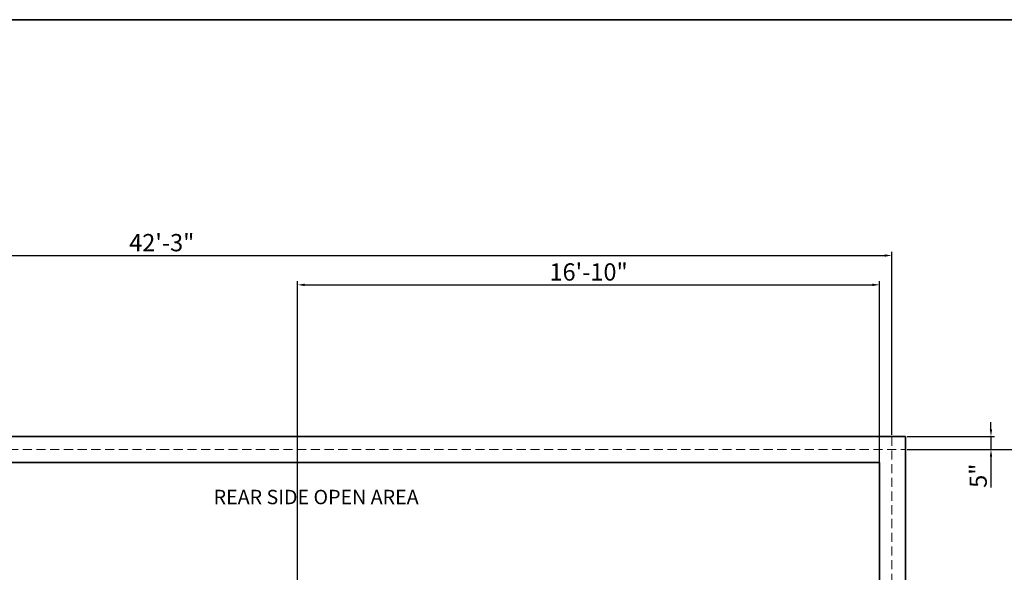
# Model space of a CAD drawing. Units: inches. Extents: x 2123 to 2977, y 1464 to 2698.
# Tile 9 of 10: x 2459 to 2801, y 2506 to 2698. Entities that reach past the tile are written whole.
import ezdxf

# ---------------------------------------------------------------- set-up
doc = ezdxf.new("R2010")
doc.units = ezdxf.units.IN
doc.linetypes.add('HIDDEN2', pattern=[4.7625, 3.175, -1.5875])
for name, color, linetype, lineweight in [('A-ANNO-DIMS', 2, 'Continuous', 18), ('A-ANNO-TTLB', 7, 'Continuous', 35), ('A-AREA-IDEN', 7, 'Continuous', 25), ('C-PROP', 21, 'HIDDEN2', 18), ('L-SITE-WALL', 7, 'Continuous', 35)]:
    doc.layers.add(name, color=color, linetype=linetype, lineweight=lineweight)
doc.styles.get("Standard").update_dxf_attribs({"font": 'arial.ttf'})
doc.dimstyles.new('ISO-25', dxfattribs={"dimtxt": 6, "dimasz": 2.5, "dimexe": 1.25, "dimexo": 0.625, "dimtad": 1, "dimdec": 0, "dimlunit": 3, "dimtxsty": 'Standard', "dimcen": 2.5, "dimadec": 0, "dimazin": 0, "dimtfac": 1, "dimtdec": 0, "dimtmove": 0, "dimatfit": 3, "dimfxl": 1, "dimarcsym": 0})

# ---------------------------------------------------------------- blocks, each defined once
blk = doc.blocks.new('*D9')
at = {"layer": 'A-ANNO-DIMS', "color": 0, "lineweight": -2, "transparency": 16777216}
for p, q in [((2767.56, 2548.37), (2808.58, 2548.37)), ((2807.33, 2545.87), (2807.33, 1686.46)), ((2767.56, 1683.96), (2808.58, 1683.96))]:
    blk.add_line(p, q, dxfattribs=at)
at = {"layer": 'A-ANNO-DIMS', "color": 0, "transparency": 16777216}
for points in [[(2806.91, 2545.87), (2807.74, 2545.87), (2807.33, 2548.37)], [(2806.91, 1686.46), (2807.74, 1686.46), (2807.33, 1683.96)]]:
    blk.add_solid(points, dxfattribs=at)
at = {"layer": 'Defpoints', "color": 0, "transparency": 16777216}
for p in [(2766.94, 2548.37), (2766.94, 1683.96), (2807.33, 1683.96)]:
    blk.add_point(p, dxfattribs=at)
at = {"layer": 'A-ANNO-DIMS', "color": 0, "transparency": 16777216, "insert": (2803.69, 2116.16), "char_height": 6, "attachment_point": 5, "rotation": 90}
blk.add_mtext("72'", dxfattribs=at)
blk = doc.blocks.new('*D10')
at = {"layer": 'A-ANNO-DIMS', "color": 0, "lineweight": -2, "transparency": 16777216}
for p, q in [((2796.59, 2555.37), (2796.59, 2557.87)), ((2767.56, 2552.87), (2797.84, 2552.87)), ((2796.59, 2552.87), (2796.59, 2548.37)), ((2767.56, 2548.37), (2797.84, 2548.37)), ((2796.59, 2545.87), (2796.59, 2535.22))]:
    blk.add_line(p, q, dxfattribs=at)
at = {"layer": 'A-ANNO-DIMS', "color": 0, "transparency": 16777216}
for points in [[(2796.18, 2555.37), (2797.01, 2555.37), (2796.59, 2552.87)], [(2796.18, 2545.87), (2797.01, 2545.87), (2796.59, 2548.37)]]:
    blk.add_solid(points, dxfattribs=at)
at = {"layer": 'Defpoints', "color": 0, "transparency": 16777216}
for p in [(2766.94, 2552.87), (2766.94, 2548.37), (2796.59, 2548.37)]:
    blk.add_point(p, dxfattribs=at)
at = {"layer": 'A-ANNO-DIMS', "color": 0, "transparency": 16777216, "insert": (2792.92, 2539.3), "char_height": 6, "attachment_point": 5, "rotation": 90}
blk.add_mtext('5"', dxfattribs=at)
blk = doc.blocks.new('*D11')
at = {"layer": 'A-ANNO-DIMS', "color": 0, "lineweight": -2, "transparency": 16777216}
for p, q in [((2255.34, 2553.5), (2255.34, 2617)), ((2257.84, 2615.75), (2759.66, 2615.75)), ((2762.16, 2553.5), (2762.16, 2617))]:
    blk.add_line(p, q, dxfattribs=at)
at = {"layer": 'A-ANNO-DIMS', "color": 0, "transparency": 16777216}
for points in [[(2257.84, 2616.16), (2257.84, 2615.33), (2255.34, 2615.75)], [(2759.66, 2616.16), (2759.66, 2615.33), (2762.16, 2615.75)]]:
    blk.add_solid(points, dxfattribs=at)
at = {"layer": 'Defpoints', "color": 0, "transparency": 16777216}
for p in [(2762.16, 2615.75), (2255.34, 2552.87), (2762.16, 2552.87)]:
    blk.add_point(p, dxfattribs=at)
at = {"layer": 'A-ANNO-DIMS', "color": 0, "transparency": 16777216, "insert": (2508.75, 2619.44), "char_height": 6, "attachment_point": 5}
blk.add_mtext('42\'-3"', dxfattribs=at)
blk = doc.blocks.new('*D57')
at = {"layer": 'A-ANNO-DIMS', "color": 0, "lineweight": -2, "transparency": 16777216}
for p, q in [((2555.89, 1805.13), (2555.89, 2606.82)), ((2558.39, 2605.57), (2755.44, 2605.57)), ((2757.94, 1805.13), (2757.94, 2606.82))]:
    blk.add_line(p, q, dxfattribs=at)
at = {"layer": 'A-ANNO-DIMS', "color": 0, "transparency": 16777216}
for points in [[(2558.39, 2605.99), (2558.39, 2605.15), (2555.89, 2605.57)], [(2755.44, 2605.99), (2755.44, 2605.15), (2757.94, 2605.57)]]:
    blk.add_solid(points, dxfattribs=at)
at = {"layer": 'Defpoints', "color": 0, "transparency": 16777216}
for p in [(2757.94, 2605.57), (2555.89, 1804.5), (2757.94, 1804.5)]:
    blk.add_point(p, dxfattribs=at)
at = {"layer": 'A-ANNO-DIMS', "color": 0, "transparency": 16777216, "insert": (2656.91, 2609.26), "char_height": 6, "attachment_point": 5}
blk.add_mtext('16\'-10"', dxfattribs=at)

msp = doc.modelspace()

# ---------------------------------------------------------------- linework, layer by layer
at = {"layer": 'A-ANNO-TTLB'}
msp.add_lwpolyline([(2123.3, 2697.62), (2977.18, 2697.62), (2977.18, 1463.53), (2123.3, 1463.53)], close=True, dxfattribs=at)
at = {"layer": 'C-PROP'}
for p, q in [((2762.16, 2552.87), (2762.16, 1683.96)), ((2250.94, 2548.37), (2766.94, 2548.37))]:
    msp.add_line(p, q, dxfattribs=at)
at = {"layer": 'L-SITE-WALL'}
for p, q in [((2766.94, 2552.87), (2250.94, 2552.87)), ((2766.94, 2425.87), (2766.94, 2552.87)), ((2757.94, 2543.87), (2259.94, 2543.87)), ((2757.94, 2425.87), (2757.94, 2543.87))]:
    msp.add_line(p, q, dxfattribs=at)

# ---------------------------------------------------------------- texts
at = {"layer": 'A-AREA-IDEN', "insert": (2526.77, 2534.41), "char_height": 5, "attachment_point": 1}
msp.add_mtext_dynamic_manual_height_columns('REAR SIDE OPEN AREA', width=209.6107, gutter_width=12.5, heights=[0], dxfattribs=at)

# ---------------------------------------------------------------- dimensions: what is measured, and where the dimension line sits
at = {"layer": 'A-ANNO-DIMS'}
for base, p1, p2, override, picture, middle in [((2762.16, 2615.75), (2255.34, 2552.87), (2762.16, 2552.87), {"dimclrd": 0, "dimclre": 0, "dimclrt": 0}, '*D11', (2508.75, 2619.44)), ((2757.9353, 2605.5708), (2555.8869, 1804.5032), (2757.9353, 1804.5032), {"dimdec": 1, "dimlfac": 1, "dimrnd": 0, "dimzin": 1, "dimdsep": 46, "dimlunit": 4, "dimfrac": 2}, '*D57', (2656.9111, 2609.2592))]:
    dim = msp.add_linear_dim(base=base, p1=p1, p2=p2, dimstyle='ISO-25', override=override, dxfattribs=at)
    dim.commit()
    dim.dimension.update_dxf_attribs({"geometry": picture, "text_midpoint": middle})
for base, p1, p2, picture, middle in [((2796.59419876, 2548.37076072), (2766.93529578, 2552.87076072), (2766.93529578, 2548.37076072), '*D10', (2792.91803914, 2539.29760247)), ((2807.33, 1683.96), (2766.94, 2548.37), (2766.94, 1683.96), '*D9', (2803.69, 2116.16))]:
    dim = msp.add_linear_dim(base=base, p1=p1, p2=p2, angle=90, dimstyle='ISO-25', override={"dimclrd": 0, "dimclre": 0, "dimclrt": 0}, dxfattribs=at)
    dim.commit()
    dim.dimension.update_dxf_attribs({"geometry": picture, "text_midpoint": middle})

doc.saveas('drawing.dxf')
